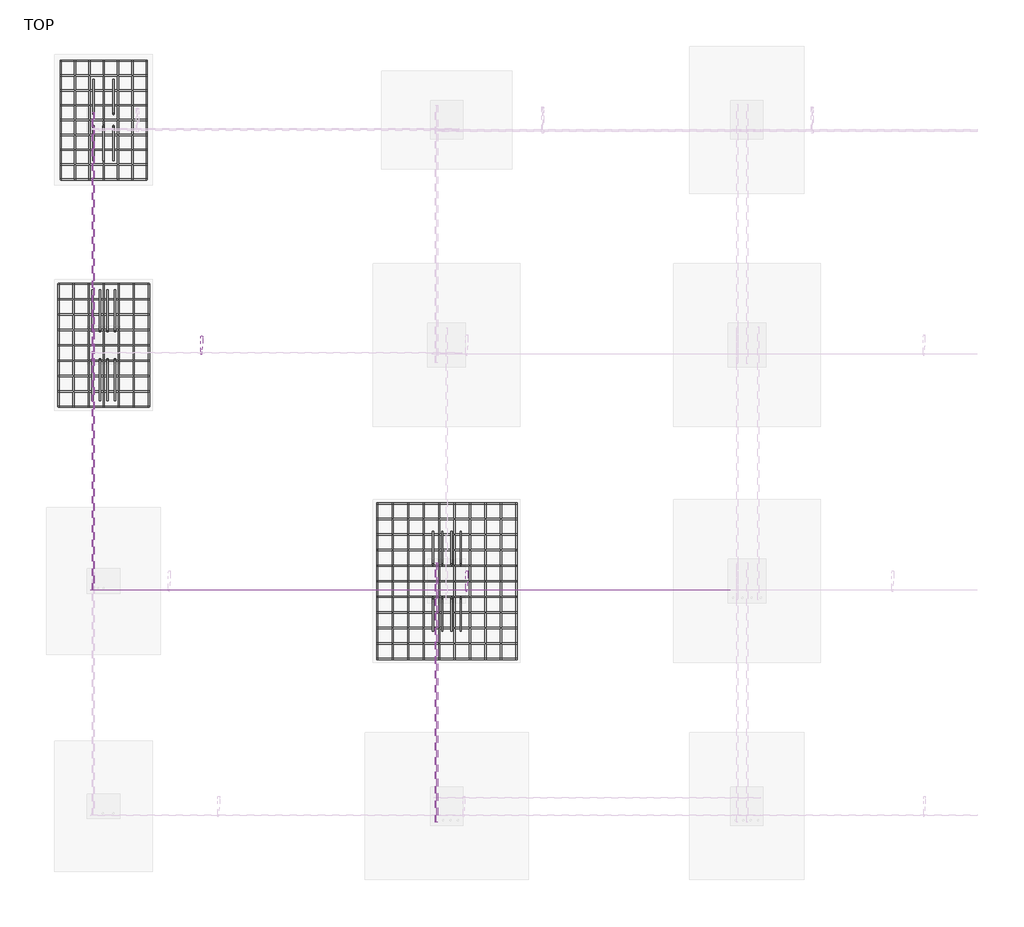
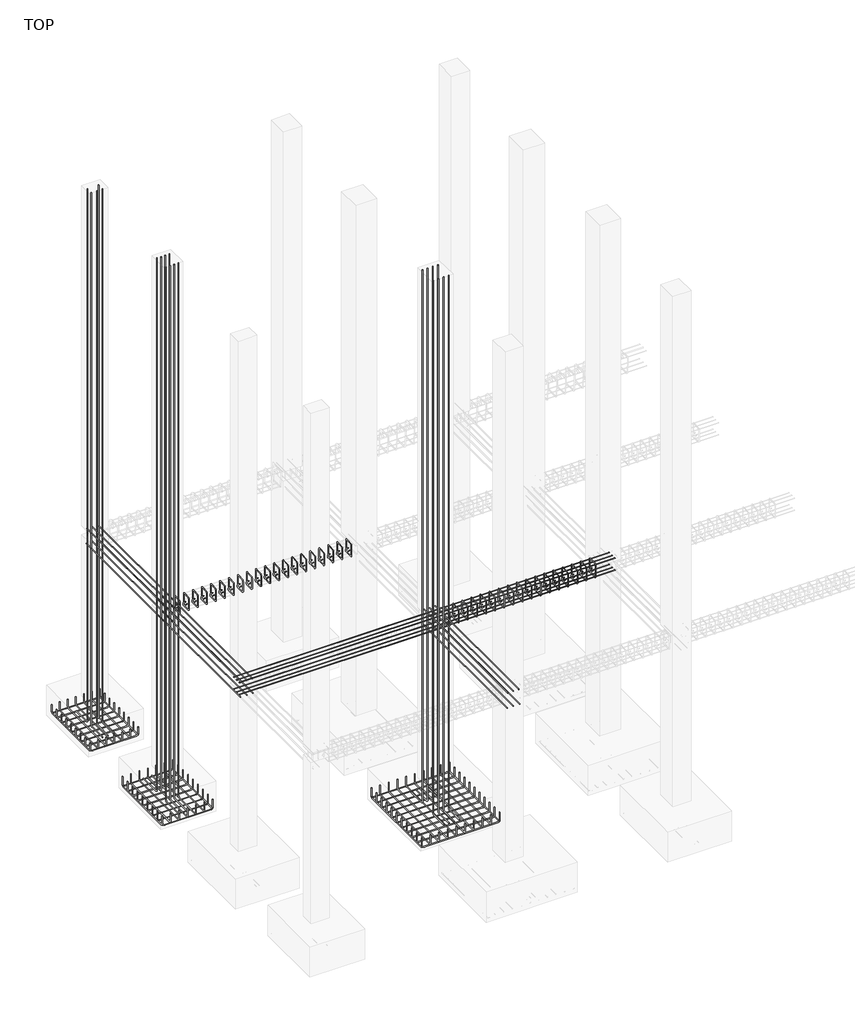
# One storey, part 3 of 8: 24 reinforcing bars.
"""IFC4 building model written with IfcOpenShell, lengths in millimetres."""

from ifc_helpers import new_model, si_unit, point, frame, origin, place, context, project, spatial, polyline, circle_curve, trimmed, segment, composite_curve, source, transform, mapped, element, save
from ifc_brep_helpers import swept_disk

model = new_model("IFC4")

# Units and contexts
model_context = context("Model", 3, world=origin())
ifc_project = project(units=[si_unit("LENGTHUNIT", "METRE", prefix="MILLI")], contexts=[model_context])

# Site, building, storey
site = spatial("IfcSite", under=ifc_project)
building = spatial("IfcBuilding", under=site)
storey = spatial("IfcBuildingStorey", under=building, Name="TOP", Elevation=0.0)

# Reinforcing bars
placement = place(None, origin())
reinforcing_bar_shape = source(origin(), model_context, "Body", "SolidModel", [
    swept_disk(composite_curve([segment(polyline([(-4763.7160601, 8075.5307576, -331.0), (-4763.7160601, 8075.5307576, -447.4)]), True, "CONTINUOUS"), segment(trimmed(circle_curve(frame((-4763.7160601, 8045.5307576, -447.4), z_axis=(-1.0, 0.0, 0.0), x_axis=(0.0, 30.0, 0.0)), 30.0), [point((-4763.7160601, 8075.5307576, -447.4))], [point((-4763.7160601, 8045.5307576, -477.4))], True, "CARTESIAN"), True, "CONTINUOUS"), segment(polyline([(-4763.7160601, 8045.5307576, -477.4), (-4763.7160601, 6998.3307576, -477.4)]), True, "CONTINUOUS"), segment(trimmed(circle_curve(frame((-4763.7160601, 6998.3307576, -447.4), z_axis=(-1.0, 0.0, 0.0), x_axis=(0.0, 0.0, -30.0)), 30.0), [point((-4763.7160601, 6998.3307576, -477.4))], [point((-4763.7160601, 6968.3307576, -447.4))], True, "CARTESIAN"), True, "CONTINUOUS"), segment(polyline([(-4763.7160601, 6968.3307576, -447.4), (-4763.7160601, 6968.3307576, -331.0)]), True, "CONTINUOUS")], self_intersect=False), 6.0),
])
element("IfcReinforcingBar", 1, at=placement, inside=storey, context=model_context, shape_type="MappedRepresentation", body=[
    mapped(reinforcing_bar_shape, transform((0.0, 0.0, 0.0), x_axis=(1.0, 0.0, 0.0), y_axis=(0.0, 1.0, 0.0), z_axis=(0.0, 0.0, 1.0))),
    mapped(reinforcing_bar_shape, transform((-133.7333333, 0.0, 0.0), x_axis=(1.0, 0.0, 0.0), y_axis=(0.0, 1.0, 0.0), z_axis=(0.0, 0.0, 1.0))),
    mapped(reinforcing_bar_shape, transform((-267.4666667, 0.0, 0.0), x_axis=(1.0, 0.0, 0.0), y_axis=(0.0, 1.0, 0.0), z_axis=(0.0, 0.0, 1.0))),
    mapped(reinforcing_bar_shape, transform((-401.2, 0.0, 0.0), x_axis=(1.0, 0.0, 0.0), y_axis=(0.0, 1.0, 0.0), z_axis=(0.0, 0.0, 1.0))),
    mapped(reinforcing_bar_shape, transform((-534.9333333, 0.0, 0.0), x_axis=(1.0, 0.0, 0.0), y_axis=(0.0, 1.0, 0.0), z_axis=(0.0, 0.0, 1.0))),
    mapped(reinforcing_bar_shape, transform((-668.6666667, 0.0, 0.0), x_axis=(1.0, 0.0, 0.0), y_axis=(0.0, 1.0, 0.0), z_axis=(0.0, 0.0, 1.0))),
    mapped(reinforcing_bar_shape, transform((-802.4, 0.0, 0.0), x_axis=(1.0, 0.0, 0.0), y_axis=(0.0, 1.0, 0.0), z_axis=(0.0, 0.0, 1.0))),
])
reinforcing_bar_2_shape = source(origin(), model_context, "Body", "SolidModel", [
    swept_disk(composite_curve([segment(polyline([(-5566.1160601, 8075.5307576, -331.0), (-5566.1160601, 8075.5307576, -447.4)]), True, "CONTINUOUS"), segment(trimmed(circle_curve(frame((-5536.1160601, 8075.5307576, -447.4), z_axis=(0.0, -1.0, 0.0), x_axis=(-30.0, 0.0, 0.0)), 30.0), [point((-5566.1160601, 8075.5307576, -447.4))], [point((-5536.1160601, 8075.5307576, -477.4))], True, "CARTESIAN"), True, "CONTINUOUS"), segment(polyline([(-5536.1160601, 8075.5307576, -477.4), (-4793.7160601, 8075.5307576, -477.4)]), True, "CONTINUOUS"), segment(trimmed(circle_curve(frame((-4793.7160601, 8075.5307576, -447.4), z_axis=(0.0, -1.0, 0.0), x_axis=(0.0, 0.0, -30.0)), 30.0), [point((-4793.7160601, 8075.5307576, -477.4))], [point((-4763.7160601, 8075.5307576, -447.4))], True, "CARTESIAN"), True, "CONTINUOUS"), segment(polyline([(-4763.7160601, 8075.5307576, -447.4), (-4763.7160601, 8075.5307576, -331.0)]), True, "CONTINUOUS")], self_intersect=False), 6.0),
])
element("IfcReinforcingBar", 2, at=placement, inside=storey, context=model_context, shape_type="MappedRepresentation", body=[
    mapped(reinforcing_bar_2_shape, transform((0.0, 0.0, 0.0), x_axis=(1.0, 0.0, 0.0), y_axis=(0.0, 1.0, 0.0), z_axis=(0.0, 0.0, 1.0))),
    mapped(reinforcing_bar_2_shape, transform((0.0, -138.4, 0.0), x_axis=(1.0, 0.0, 0.0), y_axis=(0.0, 1.0, 0.0), z_axis=(0.0, 0.0, 1.0))),
    mapped(reinforcing_bar_2_shape, transform((0.0, -276.8, 0.0), x_axis=(1.0, 0.0, 0.0), y_axis=(0.0, 1.0, 0.0), z_axis=(0.0, 0.0, 1.0))),
    mapped(reinforcing_bar_2_shape, transform((0.0, -415.2, 0.0), x_axis=(1.0, 0.0, 0.0), y_axis=(0.0, 1.0, 0.0), z_axis=(0.0, 0.0, 1.0))),
    mapped(reinforcing_bar_2_shape, transform((0.0, -553.6, 0.0), x_axis=(1.0, 0.0, 0.0), y_axis=(0.0, 1.0, 0.0), z_axis=(0.0, 0.0, 1.0))),
    mapped(reinforcing_bar_2_shape, transform((0.0, -692.0, 0.0), x_axis=(1.0, 0.0, 0.0), y_axis=(0.0, 1.0, 0.0), z_axis=(0.0, 0.0, 1.0))),
    mapped(reinforcing_bar_2_shape, transform((0.0, -830.4, 0.0), x_axis=(1.0, 0.0, 0.0), y_axis=(0.0, 1.0, 0.0), z_axis=(0.0, 0.0, 1.0))),
    mapped(reinforcing_bar_2_shape, transform((0.0, -968.8, 0.0), x_axis=(1.0, 0.0, 0.0), y_axis=(0.0, 1.0, 0.0), z_axis=(0.0, 0.0, 1.0))),
    mapped(reinforcing_bar_2_shape, transform((0.0, -1107.2, 0.0), x_axis=(1.0, 0.0, 0.0), y_axis=(0.0, 1.0, 0.0), z_axis=(0.0, 0.0, 1.0))),
])
reinforcing_bar_3_shape = source(origin(), model_context, "Body", "SolidModel", [
    swept_disk(composite_curve([segment(polyline([(-5259.3160601, 7577.9568407, 8958.464), (-5259.3160601, 7577.9568407, -415.886)]), True, "CONTINUOUS"), segment(trimmed(circle_curve(frame((-5259.3160601, 7607.9568407, -415.886), z_axis=(1.0, 0.0, 0.0), x_axis=(0.0, -30.0, 0.0)), 30.0), [point((-5259.3160601, 7577.9568407, -415.886))], [point((-5259.3160601, 7607.9568407, -445.886))], True, "CARTESIAN"), True, "CONTINUOUS"), segment(polyline([(-5259.3160601, 7607.9568407, -445.886), (-5259.3160601, 7901.0307576, -445.886)]), True, "CONTINUOUS")], self_intersect=False), 6.0),
])
element("IfcReinforcingBar", 3, at=placement, inside=storey, context=model_context, shape_type="MappedRepresentation", body=[
    mapped(reinforcing_bar_3_shape, transform((0.0, 0.0, 0.0), x_axis=(1.0, 0.0, 0.0), y_axis=(0.0, 1.0, 0.0), z_axis=(0.0, 0.0, 1.0))),
    mapped(reinforcing_bar_3_shape, transform((185.9681172, 0.0, 0.0), x_axis=(1.0, 0.0, 0.0), y_axis=(0.0, 1.0, 0.0), z_axis=(0.0, 0.0, 1.0))),
])
reinforcing_bar_4_shape = source(origin(), model_context, "Body", "SolidModel", [
    swept_disk(composite_curve([segment(polyline([(-5073.3479429, 7465.6307576, 8958.464), (-5073.3479429, 7465.6307576, -415.886)]), True, "CONTINUOUS"), segment(trimmed(circle_curve(frame((-5073.3479429, 7435.6307576, -415.886), z_axis=(-1.0, 0.0, 0.0), x_axis=(0.0, 30.0, 0.0)), 30.0), [point((-5073.3479429, 7465.6307576, -415.886))], [point((-5073.3479429, 7435.6307576, -445.886))], True, "CARTESIAN"), True, "CONTINUOUS"), segment(polyline([(-5073.3479429, 7435.6307576, -445.886), (-5073.3479429, 7142.8307576, -445.886)]), True, "CONTINUOUS")], self_intersect=False), 6.0),
])
element("IfcReinforcingBar", 4, at=placement, inside=storey, context=model_context, shape_type="MappedRepresentation", body=[
    mapped(reinforcing_bar_4_shape, transform((0.0, 0.0, 0.0), x_axis=(1.0, 0.0, 0.0), y_axis=(0.0, 1.0, 0.0), z_axis=(0.0, 0.0, 1.0))),
    mapped(reinforcing_bar_4_shape, transform((-92.9840586, 0.0, 0.0), x_axis=(1.0, 0.0, 0.0), y_axis=(0.0, 1.0, 0.0), z_axis=(0.0, 0.0, 1.0))),
    mapped(reinforcing_bar_4_shape, transform((-185.9681172, 0.0, 0.0), x_axis=(1.0, 0.0, 0.0), y_axis=(0.0, 1.0, 0.0), z_axis=(0.0, 0.0, 1.0))),
])
reinforcing_bar_5_shape = source(origin(), model_context, "Body", "SolidModel", [
    swept_disk(composite_curve([segment(polyline([(-4743.7160601, 5995.5307576, -331.0), (-4743.7160601, 5995.5307576, -467.4)]), True, "CONTINUOUS"), segment(trimmed(circle_curve(frame((-4743.7160601, 5965.5307576, -467.4), z_axis=(-1.0, 0.0, 0.0), x_axis=(0.0, 30.0, 0.0)), 30.0), [point((-4743.7160601, 5995.5307576, -467.4))], [point((-4743.7160601, 5965.5307576, -497.4))], True, "CARTESIAN"), True, "CONTINUOUS"), segment(polyline([(-4743.7160601, 5965.5307576, -497.4), (-4743.7160601, 4878.3307576, -497.4)]), True, "CONTINUOUS"), segment(trimmed(circle_curve(frame((-4743.7160601, 4878.3307576, -467.4), z_axis=(-1.0, 0.0, 0.0), x_axis=(0.0, 0.0, -30.0)), 30.0), [point((-4743.7160601, 4878.3307576, -497.4))], [point((-4743.7160601, 4848.3307576, -467.4))], True, "CARTESIAN"), True, "CONTINUOUS"), segment(polyline([(-4743.7160601, 4848.3307576, -467.4), (-4743.7160601, 4848.3307576, -331.0)]), True, "CONTINUOUS")], self_intersect=False), 6.0),
])
element("IfcReinforcingBar", 5, at=placement, inside=storey, context=model_context, shape_type="MappedRepresentation", body=[
    mapped(reinforcing_bar_5_shape, transform((0.0, 0.0, 0.0), x_axis=(1.0, 0.0, 0.0), y_axis=(0.0, 1.0, 0.0), z_axis=(0.0, 0.0, 1.0))),
    mapped(reinforcing_bar_5_shape, transform((-140.4, 0.0, 0.0), x_axis=(1.0, 0.0, 0.0), y_axis=(0.0, 1.0, 0.0), z_axis=(0.0, 0.0, 1.0))),
    mapped(reinforcing_bar_5_shape, transform((-280.8, 0.0, 0.0), x_axis=(1.0, 0.0, 0.0), y_axis=(0.0, 1.0, 0.0), z_axis=(0.0, 0.0, 1.0))),
    mapped(reinforcing_bar_5_shape, transform((-421.2, 0.0, 0.0), x_axis=(1.0, 0.0, 0.0), y_axis=(0.0, 1.0, 0.0), z_axis=(0.0, 0.0, 1.0))),
    mapped(reinforcing_bar_5_shape, transform((-561.6, 0.0, 0.0), x_axis=(1.0, 0.0, 0.0), y_axis=(0.0, 1.0, 0.0), z_axis=(0.0, 0.0, 1.0))),
    mapped(reinforcing_bar_5_shape, transform((-702.0, 0.0, 0.0), x_axis=(1.0, 0.0, 0.0), y_axis=(0.0, 1.0, 0.0), z_axis=(0.0, 0.0, 1.0))),
    mapped(reinforcing_bar_5_shape, transform((-842.4, 0.0, 0.0), x_axis=(1.0, 0.0, 0.0), y_axis=(0.0, 1.0, 0.0), z_axis=(0.0, 0.0, 1.0))),
])
reinforcing_bar_6_shape = source(origin(), model_context, "Body", "SolidModel", [
    swept_disk(composite_curve([segment(polyline([(-5586.1160601, 5995.5307576, -331.0), (-5586.1160601, 5995.5307576, -467.4)]), True, "CONTINUOUS"), segment(trimmed(circle_curve(frame((-5556.1160601, 5995.5307576, -467.4), z_axis=(0.0, -1.0, 0.0), x_axis=(-30.0, 0.0, 0.0)), 30.0), [point((-5586.1160601, 5995.5307576, -467.4))], [point((-5556.1160601, 5995.5307576, -497.4))], True, "CARTESIAN"), True, "CONTINUOUS"), segment(polyline([(-5556.1160601, 5995.5307576, -497.4), (-4773.7160601, 5995.5307576, -497.4)]), True, "CONTINUOUS"), segment(trimmed(circle_curve(frame((-4773.7160601, 5995.5307576, -467.4), z_axis=(0.0, -1.0, 0.0), x_axis=(0.0, 0.0, -30.0)), 30.0), [point((-4773.7160601, 5995.5307576, -497.4))], [point((-4743.7160601, 5995.5307576, -467.4))], True, "CARTESIAN"), True, "CONTINUOUS"), segment(polyline([(-4743.7160601, 5995.5307576, -467.4), (-4743.7160601, 5995.5307576, -331.0)]), True, "CONTINUOUS")], self_intersect=False), 6.0),
])
element("IfcReinforcingBar", 6, at=placement, inside=storey, context=model_context, shape_type="MappedRepresentation", body=[
    mapped(reinforcing_bar_6_shape, transform((0.0, 0.0, 0.0), x_axis=(1.0, 0.0, 0.0), y_axis=(0.0, 1.0, 0.0), z_axis=(0.0, 0.0, 1.0))),
    mapped(reinforcing_bar_6_shape, transform((0.0, -143.4, 0.0), x_axis=(1.0, 0.0, 0.0), y_axis=(0.0, 1.0, 0.0), z_axis=(0.0, 0.0, 1.0))),
    mapped(reinforcing_bar_6_shape, transform((0.0, -286.8, 0.0), x_axis=(1.0, 0.0, 0.0), y_axis=(0.0, 1.0, 0.0), z_axis=(0.0, 0.0, 1.0))),
    mapped(reinforcing_bar_6_shape, transform((0.0, -430.2, 0.0), x_axis=(1.0, 0.0, 0.0), y_axis=(0.0, 1.0, 0.0), z_axis=(0.0, 0.0, 1.0))),
    mapped(reinforcing_bar_6_shape, transform((0.0, -573.6, 0.0), x_axis=(1.0, 0.0, 0.0), y_axis=(0.0, 1.0, 0.0), z_axis=(0.0, 0.0, 1.0))),
    mapped(reinforcing_bar_6_shape, transform((0.0, -717.0, 0.0), x_axis=(1.0, 0.0, 0.0), y_axis=(0.0, 1.0, 0.0), z_axis=(0.0, 0.0, 1.0))),
    mapped(reinforcing_bar_6_shape, transform((0.0, -860.4, 0.0), x_axis=(1.0, 0.0, 0.0), y_axis=(0.0, 1.0, 0.0), z_axis=(0.0, 0.0, 1.0))),
    mapped(reinforcing_bar_6_shape, transform((0.0, -1003.8, 0.0), x_axis=(1.0, 0.0, 0.0), y_axis=(0.0, 1.0, 0.0), z_axis=(0.0, 0.0, 1.0))),
    mapped(reinforcing_bar_6_shape, transform((0.0, -1147.2, 0.0), x_axis=(1.0, 0.0, 0.0), y_axis=(0.0, 1.0, 0.0), z_axis=(0.0, 0.0, 1.0))),
])
reinforcing_bar_7_shape = source(origin(), model_context, "Body", "SolidModel", [
    swept_disk(composite_curve([segment(polyline([(-5269.3160601, 5551.7815576, 8968.464), (-5269.3160601, 5551.7815576, -409.536)]), True, "CONTINUOUS"), segment(trimmed(circle_curve(frame((-5269.3160601, 5581.7815576, -409.536), z_axis=(1.0, 0.0, 0.0), x_axis=(0.0, -30.0, 0.0)), 30.0), [point((-5269.3160601, 5551.7815576, -409.536))], [point((-5269.3160601, 5581.7815576, -439.536))], True, "CARTESIAN"), True, "CONTINUOUS"), segment(polyline([(-5269.3160601, 5581.7815576, -439.536), (-5269.3160601, 5940.7815576, -439.536)]), True, "CONTINUOUS")], self_intersect=False), 6.0),
])
element("IfcReinforcingBar", 7, at=placement, inside=storey, context=model_context, shape_type="MappedRepresentation", body=[
    mapped(reinforcing_bar_7_shape, transform((0.0, 0.0, 0.0), x_axis=(1.0, 0.0, 0.0), y_axis=(0.0, 1.0, 0.0), z_axis=(0.0, 0.0, 1.0))),
    mapped(reinforcing_bar_7_shape, transform((69.6, 0.0, 0.0), x_axis=(1.0, 0.0, 0.0), y_axis=(0.0, 1.0, 0.0), z_axis=(0.0, 0.0, 1.0))),
    mapped(reinforcing_bar_7_shape, transform((139.2, 0.0, 0.0), x_axis=(1.0, 0.0, 0.0), y_axis=(0.0, 1.0, 0.0), z_axis=(0.0, 0.0, 1.0))),
    mapped(reinforcing_bar_7_shape, transform((208.8, 0.0, 0.0), x_axis=(1.0, 0.0, 0.0), y_axis=(0.0, 1.0, 0.0), z_axis=(0.0, 0.0, 1.0))),
])
reinforcing_bar_8_shape = source(origin(), model_context, "Body", "SolidModel", [
    swept_disk(composite_curve([segment(polyline([(-5060.5160601, 5292.0799576, 8968.464), (-5060.5160601, 5292.0799576, -415.886)]), True, "CONTINUOUS"), segment(trimmed(circle_curve(frame((-5060.5160601, 5262.0799576, -415.886), z_axis=(-1.0, 0.0, 0.0), x_axis=(0.0, 30.0, 0.0)), 30.0), [point((-5060.5160601, 5292.0799576, -415.886))], [point((-5060.5160601, 5262.0799576, -445.886))], True, "CARTESIAN"), True, "CONTINUOUS"), segment(polyline([(-5060.5160601, 5262.0799576, -445.886), (-5060.5160601, 4903.0799576, -445.886)]), True, "CONTINUOUS")], self_intersect=False), 6.0),
])
element("IfcReinforcingBar", 8, at=placement, inside=storey, context=model_context, shape_type="MappedRepresentation", body=[
    mapped(reinforcing_bar_8_shape, transform((0.0, 0.0, 0.0), x_axis=(1.0, 0.0, 0.0), y_axis=(0.0, 1.0, 0.0), z_axis=(0.0, 0.0, 1.0))),
    mapped(reinforcing_bar_8_shape, transform((-69.6, 0.0, 0.0), x_axis=(1.0, 0.0, 0.0), y_axis=(0.0, 1.0, 0.0), z_axis=(0.0, 0.0, 1.0))),
    mapped(reinforcing_bar_8_shape, transform((-139.2, 0.0, 0.0), x_axis=(1.0, 0.0, 0.0), y_axis=(0.0, 1.0, 0.0), z_axis=(0.0, 0.0, 1.0))),
    mapped(reinforcing_bar_8_shape, transform((-208.8, 0.0, 0.0), x_axis=(1.0, 0.0, 0.0), y_axis=(0.0, 1.0, 0.0), z_axis=(0.0, 0.0, 1.0))),
])
reinforcing_bar_9_shape = source(origin(), model_context, "Body", "SolidModel", [
    swept_disk(composite_curve([segment(polyline([(-2094.7668601, 3376.2799576, 8968.464), (-2094.7668601, 3376.2799576, -403.186)]), True, "CONTINUOUS"), segment(trimmed(circle_curve(frame((-2094.7668601, 3406.2799576, -403.186), z_axis=(1.0, 0.0, 0.0), x_axis=(0.0, -30.0, 0.0)), 30.0), [point((-2094.7668601, 3376.2799576, -403.186))], [point((-2094.7668601, 3406.2799576, -433.186))], True, "CARTESIAN"), True, "CONTINUOUS"), segment(polyline([(-2094.7668601, 3406.2799576, -433.186), (-2094.7668601, 3689.0799576, -433.186)]), True, "CONTINUOUS")], self_intersect=False), 6.0),
])
element("IfcReinforcingBar", 9, at=placement, inside=storey, context=model_context, shape_type="MappedRepresentation", body=[
    mapped(reinforcing_bar_9_shape, transform((0.0, 0.0, 0.0), x_axis=(1.0, 0.0, 0.0), y_axis=(0.0, 1.0, 0.0), z_axis=(0.0, 0.0, 1.0))),
    mapped(reinforcing_bar_9_shape, transform((86.5672, 0.0, 0.0), x_axis=(1.0, 0.0, 0.0), y_axis=(0.0, 1.0, 0.0), z_axis=(0.0, 0.0, 1.0))),
    mapped(reinforcing_bar_9_shape, transform((173.1344, 0.0, 0.0), x_axis=(1.0, 0.0, 0.0), y_axis=(0.0, 1.0, 0.0), z_axis=(0.0, 0.0, 1.0))),
    mapped(reinforcing_bar_9_shape, transform((259.7016, 0.0, 0.0), x_axis=(1.0, 0.0, 0.0), y_axis=(0.0, 1.0, 0.0), z_axis=(0.0, 0.0, 1.0))),
])
reinforcing_bar_10_shape = source(origin(), model_context, "Body", "SolidModel", [
    swept_disk(composite_curve([segment(polyline([(-1835.0652601, 3065.9815576, 8968.464), (-1835.0652601, 3065.9815576, -409.536)]), True, "CONTINUOUS"), segment(trimmed(circle_curve(frame((-1835.0652601, 3035.9815576, -409.536), z_axis=(-1.0, 0.0, 0.0), x_axis=(0.0, 30.0, 0.0)), 30.0), [point((-1835.0652601, 3065.9815576, -409.536))], [point((-1835.0652601, 3035.9815576, -439.536))], True, "CARTESIAN"), True, "CONTINUOUS"), segment(polyline([(-1835.0652601, 3035.9815576, -439.536), (-1835.0652601, 2753.1815576, -439.536)]), True, "CONTINUOUS")], self_intersect=False), 6.0),
])
element("IfcReinforcingBar", 10, at=placement, inside=storey, context=model_context, shape_type="MappedRepresentation", body=[
    mapped(reinforcing_bar_10_shape, transform((0.0, 0.0, 0.0), x_axis=(1.0, 0.0, 0.0), y_axis=(0.0, 1.0, 0.0), z_axis=(0.0, 0.0, 1.0))),
    mapped(reinforcing_bar_10_shape, transform((-86.5672, 0.0, 0.0), x_axis=(1.0, 0.0, 0.0), y_axis=(0.0, 1.0, 0.0), z_axis=(0.0, 0.0, 1.0))),
    mapped(reinforcing_bar_10_shape, transform((-173.1344, 0.0, 0.0), x_axis=(1.0, 0.0, 0.0), y_axis=(0.0, 1.0, 0.0), z_axis=(0.0, 0.0, 1.0))),
    mapped(reinforcing_bar_10_shape, transform((-259.7016, 0.0, 0.0), x_axis=(1.0, 0.0, 0.0), y_axis=(0.0, 1.0, 0.0), z_axis=(0.0, 0.0, 1.0))),
])
reinforcing_bar_11_shape = source(origin(), model_context, "Body", "SolidModel", [
    swept_disk(composite_curve([segment(polyline([(-2614.7160601, 3947.1307576, -331.0), (-2614.7160601, 3947.1307576, -467.4)]), True, "CONTINUOUS"), segment(trimmed(circle_curve(frame((-2584.7160601, 3947.1307576, -467.4), z_axis=(0.0, -1.0, 0.0), x_axis=(-30.0, 0.0, 0.0)), 30.0), [point((-2614.7160601, 3947.1307576, -467.4))], [point((-2584.7160601, 3947.1307576, -497.4))], True, "CARTESIAN"), True, "CONTINUOUS"), segment(polyline([(-2584.7160601, 3947.1307576, -497.4), (-1345.1160601, 3947.1307576, -497.4)]), True, "CONTINUOUS"), segment(trimmed(circle_curve(frame((-1345.1160601, 3947.1307576, -467.4), z_axis=(0.0, -1.0, 0.0), x_axis=(0.0, 0.0, -30.0)), 30.0), [point((-1345.1160601, 3947.1307576, -497.4))], [point((-1315.1160601, 3947.1307576, -467.4))], True, "CARTESIAN"), True, "CONTINUOUS"), segment(polyline([(-1315.1160601, 3947.1307576, -467.4), (-1315.1160601, 3947.1307576, -331.0)]), True, "CONTINUOUS")], self_intersect=False), 6.0),
])
element("IfcReinforcingBar", 11, at=placement, inside=storey, context=model_context, shape_type="MappedRepresentation", body=[
    mapped(reinforcing_bar_11_shape, transform((0.0, 0.0, 0.0), x_axis=(1.0, 0.0, 0.0), y_axis=(0.0, 1.0, 0.0), z_axis=(0.0, 0.0, 1.0))),
    mapped(reinforcing_bar_11_shape, transform((0.0, -145.2, 0.0), x_axis=(1.0, 0.0, 0.0), y_axis=(0.0, 1.0, 0.0), z_axis=(0.0, 0.0, 1.0))),
    mapped(reinforcing_bar_11_shape, transform((0.0, -290.4, 0.0), x_axis=(1.0, 0.0, 0.0), y_axis=(0.0, 1.0, 0.0), z_axis=(0.0, 0.0, 1.0))),
    mapped(reinforcing_bar_11_shape, transform((0.0, -435.6, 0.0), x_axis=(1.0, 0.0, 0.0), y_axis=(0.0, 1.0, 0.0), z_axis=(0.0, 0.0, 1.0))),
    mapped(reinforcing_bar_11_shape, transform((0.0, -580.8, 0.0), x_axis=(1.0, 0.0, 0.0), y_axis=(0.0, 1.0, 0.0), z_axis=(0.0, 0.0, 1.0))),
    mapped(reinforcing_bar_11_shape, transform((0.0, -726.0, 0.0), x_axis=(1.0, 0.0, 0.0), y_axis=(0.0, 1.0, 0.0), z_axis=(0.0, 0.0, 1.0))),
    mapped(reinforcing_bar_11_shape, transform((0.0, -871.2, 0.0), x_axis=(1.0, 0.0, 0.0), y_axis=(0.0, 1.0, 0.0), z_axis=(0.0, 0.0, 1.0))),
    mapped(reinforcing_bar_11_shape, transform((0.0, -1016.4, 0.0), x_axis=(1.0, 0.0, 0.0), y_axis=(0.0, 1.0, 0.0), z_axis=(0.0, 0.0, 1.0))),
    mapped(reinforcing_bar_11_shape, transform((0.0, -1161.6, 0.0), x_axis=(1.0, 0.0, 0.0), y_axis=(0.0, 1.0, 0.0), z_axis=(0.0, 0.0, 1.0))),
    mapped(reinforcing_bar_11_shape, transform((0.0, -1306.8, 0.0), x_axis=(1.0, 0.0, 0.0), y_axis=(0.0, 1.0, 0.0), z_axis=(0.0, 0.0, 1.0))),
    mapped(reinforcing_bar_11_shape, transform((0.0, -1452.0, 0.0), x_axis=(1.0, 0.0, 0.0), y_axis=(0.0, 1.0, 0.0), z_axis=(0.0, 0.0, 1.0))),
])
reinforcing_bar_12_shape = source(origin(), model_context, "Body", "SolidModel", [
    swept_disk(composite_curve([segment(polyline([(-2614.7160601, 2495.1307576, -331.0), (-2614.7160601, 2495.1307576, -467.4)]), True, "CONTINUOUS"), segment(trimmed(circle_curve(frame((-2614.7160601, 2525.1307576, -467.4), z_axis=(1.0, 0.0, 0.0), x_axis=(0.0, -30.0, 0.0)), 30.0), [point((-2614.7160601, 2495.1307576, -467.4))], [point((-2614.7160601, 2525.1307576, -497.4))], True, "CARTESIAN"), True, "CONTINUOUS"), segment(polyline([(-2614.7160601, 2525.1307576, -497.4), (-2614.7160601, 3917.1307576, -497.4)]), True, "CONTINUOUS"), segment(trimmed(circle_curve(frame((-2614.7160601, 3917.1307576, -467.4), z_axis=(1.0, 0.0, 0.0), x_axis=(0.0, 0.0, -30.0)), 30.0), [point((-2614.7160601, 3917.1307576, -497.4))], [point((-2614.7160601, 3947.1307576, -467.4))], True, "CARTESIAN"), True, "CONTINUOUS"), segment(polyline([(-2614.7160601, 3947.1307576, -467.4), (-2614.7160601, 3947.1307576, -331.0)]), True, "CONTINUOUS")], self_intersect=False), 6.0),
])
element("IfcReinforcingBar", 12, at=placement, inside=storey, context=model_context, shape_type="MappedRepresentation", body=[
    mapped(reinforcing_bar_12_shape, transform((0.0, 0.0, 0.0), x_axis=(1.0, 0.0, 0.0), y_axis=(0.0, 1.0, 0.0), z_axis=(0.0, 0.0, 1.0))),
    mapped(reinforcing_bar_12_shape, transform((144.4, 0.0, 0.0), x_axis=(1.0, 0.0, 0.0), y_axis=(0.0, 1.0, 0.0), z_axis=(0.0, 0.0, 1.0))),
    mapped(reinforcing_bar_12_shape, transform((288.8, 0.0, 0.0), x_axis=(1.0, 0.0, 0.0), y_axis=(0.0, 1.0, 0.0), z_axis=(0.0, 0.0, 1.0))),
    mapped(reinforcing_bar_12_shape, transform((433.2, 0.0, 0.0), x_axis=(1.0, 0.0, 0.0), y_axis=(0.0, 1.0, 0.0), z_axis=(0.0, 0.0, 1.0))),
    mapped(reinforcing_bar_12_shape, transform((577.6, 0.0, 0.0), x_axis=(1.0, 0.0, 0.0), y_axis=(0.0, 1.0, 0.0), z_axis=(0.0, 0.0, 1.0))),
    mapped(reinforcing_bar_12_shape, transform((722.0, 0.0, 0.0), x_axis=(1.0, 0.0, 0.0), y_axis=(0.0, 1.0, 0.0), z_axis=(0.0, 0.0, 1.0))),
    mapped(reinforcing_bar_12_shape, transform((866.4, 0.0, 0.0), x_axis=(1.0, 0.0, 0.0), y_axis=(0.0, 1.0, 0.0), z_axis=(0.0, 0.0, 1.0))),
    mapped(reinforcing_bar_12_shape, transform((1010.8, 0.0, 0.0), x_axis=(1.0, 0.0, 0.0), y_axis=(0.0, 1.0, 0.0), z_axis=(0.0, 0.0, 1.0))),
    mapped(reinforcing_bar_12_shape, transform((1155.2, 0.0, 0.0), x_axis=(1.0, 0.0, 0.0), y_axis=(0.0, 1.0, 0.0), z_axis=(0.0, 0.0, 1.0))),
    mapped(reinforcing_bar_12_shape, transform((1299.6, 0.0, 0.0), x_axis=(1.0, 0.0, 0.0), y_axis=(0.0, 1.0, 0.0), z_axis=(0.0, 0.0, 1.0))),
])
reinforcing_bar_13_shape = source(origin(), model_context, "Body", "SolidModel", [
    swept_disk(composite_curve([segment(polyline([(-5267.9226618, 7596.2307576, 2693.6917983), (-5267.9226618, 5274.0799576, 2693.6917983)]), True, "CONTINUOUS")], self_intersect=False), 5.0),
])
element("IfcReinforcingBar", 13, at=placement, inside=storey, context=model_context, shape_type="MappedRepresentation", body=[
    mapped(reinforcing_bar_13_shape, transform((0.0, 0.0, 0.0), x_axis=(1.0, 0.0, 0.0), y_axis=(0.0, 1.0, 0.0), z_axis=(0.0, 0.0, 1.0))),
    mapped(reinforcing_bar_13_shape, transform((103.0066017, 0.0, 0.0), x_axis=(1.0, 0.0, 0.0), y_axis=(0.0, 1.0, 0.0), z_axis=(0.0, 0.0, 1.0))),
    mapped(reinforcing_bar_13_shape, transform((206.0132034, 0.0, 0.0), x_axis=(1.0, 0.0, 0.0), y_axis=(0.0, 1.0, 0.0), z_axis=(0.0, 0.0, 1.0))),
])
reinforcing_bar_14_shape = source(origin(), model_context, "Body", "SolidModel", [
    swept_disk(composite_curve([segment(polyline([(-5257.3160601, 5274.0799576, 2955.0), (-5257.3160601, 7596.2307576, 2955.0)]), True, "CONTINUOUS")], self_intersect=False), 5.0),
])
element("IfcReinforcingBar", 14, at=placement, inside=storey, context=model_context, shape_type="MappedRepresentation", body=[
    mapped(reinforcing_bar_14_shape, transform((0.0, 0.0, 0.0), x_axis=(1.0, 0.0, 0.0), y_axis=(0.0, 1.0, 0.0), z_axis=(0.0, 0.0, 1.0))),
    mapped(reinforcing_bar_14_shape, transform((92.4, 0.0, 0.0), x_axis=(1.0, 0.0, 0.0), y_axis=(0.0, 1.0, 0.0), z_axis=(0.0, 0.0, 1.0))),
    mapped(reinforcing_bar_14_shape, transform((184.8, 0.0, 0.0), x_axis=(1.0, 0.0, 0.0), y_axis=(0.0, 1.0, 0.0), z_axis=(0.0, 0.0, 1.0))),
])
reinforcing_bar_15_shape = source(origin(), model_context, "Body", "SolidModel", [
    swept_disk(composite_curve([segment(polyline([(-5267.9226618, 5569.7815576, 2693.6917983), (-5267.9226618, 3136.8307576, 2693.6917983)]), True, "CONTINUOUS")], self_intersect=False), 5.0),
])
element("IfcReinforcingBar", 15, at=placement, inside=storey, context=model_context, shape_type="MappedRepresentation", body=[
    mapped(reinforcing_bar_15_shape, transform((0.0, 0.0, 0.0), x_axis=(1.0, 0.0, 0.0), y_axis=(0.0, 1.0, 0.0), z_axis=(0.0, 0.0, 1.0))),
    mapped(reinforcing_bar_15_shape, transform((103.0066017, 0.0, 0.0), x_axis=(1.0, 0.0, 0.0), y_axis=(0.0, 1.0, 0.0), z_axis=(0.0, 0.0, 1.0))),
    mapped(reinforcing_bar_15_shape, transform((206.0132034, 0.0, 0.0), x_axis=(1.0, 0.0, 0.0), y_axis=(0.0, 1.0, 0.0), z_axis=(0.0, 0.0, 1.0))),
])
reinforcing_bar_16_shape = source(origin(), model_context, "Body", "SolidModel", [
    swept_disk(composite_curve([segment(polyline([(-5257.3160601, 3136.8307576, 2955.0), (-5257.3160601, 5569.7815576, 2955.0)]), True, "CONTINUOUS")], self_intersect=False), 5.0),
])
element("IfcReinforcingBar", 16, at=placement, inside=storey, context=model_context, shape_type="MappedRepresentation", body=[
    mapped(reinforcing_bar_16_shape, transform((0.0, 0.0, 0.0), x_axis=(1.0, 0.0, 0.0), y_axis=(0.0, 1.0, 0.0), z_axis=(0.0, 0.0, 1.0))),
    mapped(reinforcing_bar_16_shape, transform((92.4, 0.0, 0.0), x_axis=(1.0, 0.0, 0.0), y_axis=(0.0, 1.0, 0.0), z_axis=(0.0, 0.0, 1.0))),
    mapped(reinforcing_bar_16_shape, transform((184.8, 0.0, 0.0), x_axis=(1.0, 0.0, 0.0), y_axis=(0.0, 1.0, 0.0), z_axis=(0.0, 0.0, 1.0))),
])
reinforcing_bar_17_shape = source(origin(), model_context, "Body", "SolidModel", [
    swept_disk(composite_curve([segment(polyline([(-2067.9226618, 3394.2799576, 2693.6917983), (-2067.9226618, 973.2799576, 2693.6917983)]), True, "CONTINUOUS")], self_intersect=False), 5.0),
])
element("IfcReinforcingBar", 17, at=placement, inside=storey, context=model_context, shape_type="MappedRepresentation", body=[
    mapped(reinforcing_bar_17_shape, transform((0.0, 0.0, 0.0), x_axis=(1.0, 0.0, 0.0), y_axis=(0.0, 1.0, 0.0), z_axis=(0.0, 0.0, 1.0))),
    mapped(reinforcing_bar_17_shape, transform((103.0066017, 0.0, 0.0), x_axis=(1.0, 0.0, 0.0), y_axis=(0.0, 1.0, 0.0), z_axis=(0.0, 0.0, 1.0))),
    mapped(reinforcing_bar_17_shape, transform((206.0132034, 0.0, 0.0), x_axis=(1.0, 0.0, 0.0), y_axis=(0.0, 1.0, 0.0), z_axis=(0.0, 0.0, 1.0))),
])
reinforcing_bar_18_shape = source(origin(), model_context, "Body", "SolidModel", [
    swept_disk(composite_curve([segment(polyline([(-2057.3160601, 973.2799576, 2955.0), (-2057.3160601, 3394.2799576, 2955.0)]), True, "CONTINUOUS")], self_intersect=False), 5.0),
])
element("IfcReinforcingBar", 18, at=placement, inside=storey, context=model_context, shape_type="MappedRepresentation", body=[
    mapped(reinforcing_bar_18_shape, transform((0.0, 0.0, 0.0), x_axis=(1.0, 0.0, 0.0), y_axis=(0.0, 1.0, 0.0), z_axis=(0.0, 0.0, 1.0))),
    mapped(reinforcing_bar_18_shape, transform((92.4, 0.0, 0.0), x_axis=(1.0, 0.0, 0.0), y_axis=(0.0, 1.0, 0.0), z_axis=(0.0, 0.0, 1.0))),
    mapped(reinforcing_bar_18_shape, transform((184.8, 0.0, 0.0), x_axis=(1.0, 0.0, 0.0), y_axis=(0.0, 1.0, 0.0), z_axis=(0.0, 0.0, 1.0))),
])
reinforcing_bar_19_shape = source(origin(), model_context, "Body", "SolidModel", [
    swept_disk(composite_curve([segment(polyline([(-2146.7668601, 5434.6753761, 2837.6888527), (-2146.7668601, 5499.0220932, 2773.3421356)]), True, "CONTINUOUS"), segment(trimmed(circle_curve(frame((-2146.7668601, 5484.8799576, 2759.2), z_axis=(-1.0, 0.0, 0.0), x_axis=(0.0, 14.142135600000074, 14.142135600000074)), 20.0), [point((-2146.7668601, 5499.0220932, 2773.3421356))], [point((-2146.7668601, 5484.8799576, 2739.2))], True, "CARTESIAN"), True, "CONTINUOUS"), segment(polyline([(-2146.7668601, 5484.8799576, 2739.2), (-2146.7668601, 5358.9815576, 2739.2)]), True, "CONTINUOUS"), segment(trimmed(circle_curve(frame((-2146.7668601, 5358.9815576, 2759.2), z_axis=(-1.0, 0.0, 0.0), x_axis=(0.0, 0.0, -20.0)), 20.0), [point((-2146.7668601, 5358.9815576, 2739.2))], [point((-2146.7668601, 5338.9815576, 2759.2))], True, "CARTESIAN"), True, "CONTINUOUS"), segment(polyline([(-2146.7668601, 5338.9815576, 2759.2), (-2146.7668601, 5338.9815576, 2936.0)]), True, "CONTINUOUS"), segment(trimmed(circle_curve(frame((-2145.8035337, 5358.9583442, 2936.0), z_axis=(-0.9988393294590433, 0.04816631526086278, 0.0), x_axis=(-0.9633263999999144, -19.976786600000196, 0.0)), 20.0), [point((-2146.7668601, 5338.9815576, 2936.0))], [point((-2145.8035337, 5358.9583442, 2956.0))], True, "CARTESIAN"), True, "CONTINUOUS"), segment(polyline([(-2145.8035337, 5358.9583442, 2956.0), (-2139.7301864, 5484.903171, 2956.0)]), True, "CONTINUOUS"), segment(trimmed(circle_curve(frame((-2139.7301864, 5484.903171, 2936.0), z_axis=(-0.9988393294590433, 0.04816631526086278, 0.0), x_axis=(0.0, 0.0, 20.0)), 20.0), [point((-2139.7301864, 5484.903171, 2956.0))], [point((-2138.7668601, 5504.8799576, 2936.0))], True, "CARTESIAN"), True, "CONTINUOUS"), segment(polyline([(-2138.7668601, 5504.8799576, 2936.0), (-2138.7668601, 5504.8799576, 2759.2)]), True, "CONTINUOUS"), segment(trimmed(circle_curve(frame((-2138.7668601, 5484.8799576, 2759.2), z_axis=(-1.0, 0.0, 0.0), x_axis=(0.0, 20.0, 0.0)), 20.0), [point((-2138.7668601, 5504.8799576, 2759.2))], [point((-2138.7668601, 5470.737822, 2745.0578644))], True, "CARTESIAN"), True, "CONTINUOUS"), segment(polyline([(-2138.7668601, 5470.737822, 2745.0578644), (-2138.7668601, 5406.3911049, 2809.4045815)]), True, "CONTINUOUS")], self_intersect=False), 4.0),
])
element("IfcReinforcingBar", 19, at=placement, inside=storey, context=model_context, shape_type="MappedRepresentation", body=[
    mapped(reinforcing_bar_19_shape, transform((0.0, 0.0, 0.0), x_axis=(1.0, 0.0, 0.0), y_axis=(0.0, 1.0, 0.0), z_axis=(0.0, 0.0, 1.0))),
    mapped(reinforcing_bar_19_shape, transform((-150.6183789, 0.0, 0.0), x_axis=(1.0, 0.0, 0.0), y_axis=(0.0, 1.0, 0.0), z_axis=(0.0, 0.0, 1.0))),
    mapped(reinforcing_bar_19_shape, transform((-301.2367579, 0.0, 0.0), x_axis=(1.0, 0.0, 0.0), y_axis=(0.0, 1.0, 0.0), z_axis=(0.0, 0.0, 1.0))),
    mapped(reinforcing_bar_19_shape, transform((-451.8551368, 0.0, 0.0), x_axis=(1.0, 0.0, 0.0), y_axis=(0.0, 1.0, 0.0), z_axis=(0.0, 0.0, 1.0))),
    mapped(reinforcing_bar_19_shape, transform((-602.4735158, 0.0, 0.0), x_axis=(1.0, 0.0, 0.0), y_axis=(0.0, 1.0, 0.0), z_axis=(0.0, 0.0, 1.0))),
    mapped(reinforcing_bar_19_shape, transform((-753.0918947, 0.0, 0.0), x_axis=(1.0, 0.0, 0.0), y_axis=(0.0, 1.0, 0.0), z_axis=(0.0, 0.0, 1.0))),
    mapped(reinforcing_bar_19_shape, transform((-903.7102737, 0.0, 0.0), x_axis=(1.0, 0.0, 0.0), y_axis=(0.0, 1.0, 0.0), z_axis=(0.0, 0.0, 1.0))),
    mapped(reinforcing_bar_19_shape, transform((-1054.3286526, 0.0, 0.0), x_axis=(1.0, 0.0, 0.0), y_axis=(0.0, 1.0, 0.0), z_axis=(0.0, 0.0, 1.0))),
    mapped(reinforcing_bar_19_shape, transform((-1204.9470316, 0.0, 0.0), x_axis=(1.0, 0.0, 0.0), y_axis=(0.0, 1.0, 0.0), z_axis=(0.0, 0.0, 1.0))),
    mapped(reinforcing_bar_19_shape, transform((-1355.5654105, 0.0, 0.0), x_axis=(1.0, 0.0, 0.0), y_axis=(0.0, 1.0, 0.0), z_axis=(0.0, 0.0, 1.0))),
    mapped(reinforcing_bar_19_shape, transform((-1506.1837895, 0.0, 0.0), x_axis=(1.0, 0.0, 0.0), y_axis=(0.0, 1.0, 0.0), z_axis=(0.0, 0.0, 1.0))),
    mapped(reinforcing_bar_19_shape, transform((-1656.8021684, 0.0, 0.0), x_axis=(1.0, 0.0, 0.0), y_axis=(0.0, 1.0, 0.0), z_axis=(0.0, 0.0, 1.0))),
    mapped(reinforcing_bar_19_shape, transform((-1807.4205474, 0.0, 0.0), x_axis=(1.0, 0.0, 0.0), y_axis=(0.0, 1.0, 0.0), z_axis=(0.0, 0.0, 1.0))),
    mapped(reinforcing_bar_19_shape, transform((-1958.0389263, 0.0, 0.0), x_axis=(1.0, 0.0, 0.0), y_axis=(0.0, 1.0, 0.0), z_axis=(0.0, 0.0, 1.0))),
    mapped(reinforcing_bar_19_shape, transform((-2108.6573053, 0.0, 0.0), x_axis=(1.0, 0.0, 0.0), y_axis=(0.0, 1.0, 0.0), z_axis=(0.0, 0.0, 1.0))),
    mapped(reinforcing_bar_19_shape, transform((-2259.2756842, 0.0, 0.0), x_axis=(1.0, 0.0, 0.0), y_axis=(0.0, 1.0, 0.0), z_axis=(0.0, 0.0, 1.0))),
    mapped(reinforcing_bar_19_shape, transform((-2409.8940632, 0.0, 0.0), x_axis=(1.0, 0.0, 0.0), y_axis=(0.0, 1.0, 0.0), z_axis=(0.0, 0.0, 1.0))),
    mapped(reinforcing_bar_19_shape, transform((-2560.5124421, 0.0, 0.0), x_axis=(1.0, 0.0, 0.0), y_axis=(0.0, 1.0, 0.0), z_axis=(0.0, 0.0, 1.0))),
    mapped(reinforcing_bar_19_shape, transform((-2711.1308211, 0.0, 0.0), x_axis=(1.0, 0.0, 0.0), y_axis=(0.0, 1.0, 0.0), z_axis=(0.0, 0.0, 1.0))),
    mapped(reinforcing_bar_19_shape, transform((-2861.7492, 0.0, 0.0), x_axis=(1.0, 0.0, 0.0), y_axis=(0.0, 1.0, 0.0), z_axis=(0.0, 0.0, 1.0))),
])
reinforcing_bar_20_shape = source(origin(), model_context, "Body", "SolidModel", [
    swept_disk(composite_curve([segment(polyline([(-1817.0652601, 3139.6962762, 2954.4852814), (-5287.3160601, 3139.6962762, 2954.4852814)]), True, "CONTINUOUS")], self_intersect=False), 4.0),
])
element("IfcReinforcingBar", 20, at=placement, inside=storey, context=model_context, shape_type="MappedRepresentation", body=[
    mapped(reinforcing_bar_20_shape, transform((0.0, 0.0, 0.0), x_axis=(1.0, 0.0, 0.0), y_axis=(0.0, 1.0, 0.0), z_axis=(0.0, 0.0, 1.0))),
    mapped(reinforcing_bar_20_shape, transform((0.0, 81.4344814, 0.0), x_axis=(1.0, 0.0, 0.0), y_axis=(0.0, 1.0, 0.0), z_axis=(0.0, 0.0, 1.0))),
    mapped(reinforcing_bar_20_shape, transform((0.0, 162.8689627, 0.0), x_axis=(1.0, 0.0, 0.0), y_axis=(0.0, 1.0, 0.0), z_axis=(0.0, 0.0, 1.0))),
])
reinforcing_bar_21_shape = source(origin(), model_context, "Body", "SolidModel", [
    swept_disk(composite_curve([segment(polyline([(-1817.0652601, 3302.565239, 2740.7147186), (-5287.3160601, 3302.565239, 2740.7147186)]), True, "CONTINUOUS")], self_intersect=False), 4.0),
])
element("IfcReinforcingBar", 21, at=placement, inside=storey, context=model_context, shape_type="MappedRepresentation", body=[
    mapped(reinforcing_bar_21_shape, transform((0.0, 0.0, 0.0), x_axis=(1.0, 0.0, 0.0), y_axis=(0.0, 1.0, 0.0), z_axis=(0.0, 0.0, 1.0))),
    mapped(reinforcing_bar_21_shape, transform((0.0, -81.4344814, 0.0), x_axis=(1.0, 0.0, 0.0), y_axis=(0.0, 1.0, 0.0), z_axis=(0.0, 0.0, 1.0))),
    mapped(reinforcing_bar_21_shape, transform((0.0, -162.8689627, 0.0), x_axis=(1.0, 0.0, 0.0), y_axis=(0.0, 1.0, 0.0), z_axis=(0.0, 0.0, 1.0))),
])
reinforcing_bar_22_shape = source(origin(), model_context, "Body", "SolidModel", [
    swept_disk(composite_curve([segment(polyline([(653.2331399, 3243.8753761, 2827.6888527), (653.2331399, 3308.2220932, 2763.3421356)]), True, "CONTINUOUS"), segment(trimmed(circle_curve(frame((653.2331399, 3294.0799576, 2749.2), z_axis=(-1.0, 0.0, 0.0), x_axis=(0.0, 14.142135600000074, 14.142135600000074)), 20.0), [point((653.2331399, 3308.2220932, 2763.3421356))], [point((653.2331399, 3294.0799576, 2729.2))], True, "CARTESIAN"), True, "CONTINUOUS"), segment(polyline([(653.2331399, 3294.0799576, 2729.2), (653.2331399, 3148.1815576, 2729.2)]), True, "CONTINUOUS"), segment(trimmed(circle_curve(frame((653.2331399, 3148.1815576, 2749.2), z_axis=(-1.0, 0.0, 0.0), x_axis=(0.0, 0.0, -20.0)), 20.0), [point((653.2331399, 3148.1815576, 2729.2))], [point((653.2331399, 3128.1815576, 2749.2))], True, "CARTESIAN"), True, "CONTINUOUS"), segment(polyline([(653.2331399, 3128.1815576, 2749.2), (653.2331399, 3128.1815576, 2946.0)]), True, "CONTINUOUS"), segment(trimmed(circle_curve(frame((654.0930293, 3148.1630638, 2946.0), z_axis=(-0.9990753104108542, 0.04299446624224492, 0.0), x_axis=(-0.8598894000000428, -19.98150620000024, 0.0)), 20.0), [point((653.2331399, 3128.1815576, 2946.0))], [point((654.0930293, 3148.1630638, 2966.0))], True, "CARTESIAN"), True, "CONTINUOUS"), segment(polyline([(654.0930293, 3148.1630638, 2966.0), (660.3732506, 3294.0984514, 2966.0)]), True, "CONTINUOUS"), segment(trimmed(circle_curve(frame((660.3732506, 3294.0984514, 2946.0), z_axis=(-0.9990753104108542, 0.04299446624224492, 0.0), x_axis=(0.0, 0.0, 20.0)), 20.0), [point((660.3732506, 3294.0984514, 2966.0))], [point((661.2331399, 3314.0799576, 2946.0))], True, "CARTESIAN"), True, "CONTINUOUS"), segment(polyline([(661.2331399, 3314.0799576, 2946.0), (661.2331399, 3314.0799576, 2749.2)]), True, "CONTINUOUS"), segment(trimmed(circle_curve(frame((661.2331399, 3294.0799576, 2749.2), z_axis=(-1.0, 0.0, 0.0), x_axis=(0.0, 20.0, 0.0)), 20.0), [point((661.2331399, 3314.0799576, 2749.2))], [point((661.2331399, 3279.937822, 2735.0578644))], True, "CARTESIAN"), True, "CONTINUOUS"), segment(polyline([(661.2331399, 3279.937822, 2735.0578644), (661.2331399, 3215.5911049, 2799.4045815)]), True, "CONTINUOUS")], self_intersect=False), 4.0),
])
element("IfcReinforcingBar", 22, at=placement, inside=storey, context=model_context, shape_type="MappedRepresentation", body=[
    mapped(reinforcing_bar_22_shape, transform((0.0, 0.0, 0.0), x_axis=(1.0, 0.0, 0.0), y_axis=(0.0, 1.0, 0.0), z_axis=(0.0, 0.0, 1.0))),
    mapped(reinforcing_bar_22_shape, transform((-152.296825, 0.0, 0.0), x_axis=(1.0, 0.0, 0.0), y_axis=(0.0, 1.0, 0.0), z_axis=(0.0, 0.0, 1.0))),
    mapped(reinforcing_bar_22_shape, transform((-304.59365, 0.0, 0.0), x_axis=(1.0, 0.0, 0.0), y_axis=(0.0, 1.0, 0.0), z_axis=(0.0, 0.0, 1.0))),
    mapped(reinforcing_bar_22_shape, transform((-456.890475, 0.0, 0.0), x_axis=(1.0, 0.0, 0.0), y_axis=(0.0, 1.0, 0.0), z_axis=(0.0, 0.0, 1.0))),
    mapped(reinforcing_bar_22_shape, transform((-609.1873, 0.0, 0.0), x_axis=(1.0, 0.0, 0.0), y_axis=(0.0, 1.0, 0.0), z_axis=(0.0, 0.0, 1.0))),
    mapped(reinforcing_bar_22_shape, transform((-761.484125, 0.0, 0.0), x_axis=(1.0, 0.0, 0.0), y_axis=(0.0, 1.0, 0.0), z_axis=(0.0, 0.0, 1.0))),
    mapped(reinforcing_bar_22_shape, transform((-913.78095, 0.0, 0.0), x_axis=(1.0, 0.0, 0.0), y_axis=(0.0, 1.0, 0.0), z_axis=(0.0, 0.0, 1.0))),
    mapped(reinforcing_bar_22_shape, transform((-1066.077775, 0.0, 0.0), x_axis=(1.0, 0.0, 0.0), y_axis=(0.0, 1.0, 0.0), z_axis=(0.0, 0.0, 1.0))),
    mapped(reinforcing_bar_22_shape, transform((-1218.3746, 0.0, 0.0), x_axis=(1.0, 0.0, 0.0), y_axis=(0.0, 1.0, 0.0), z_axis=(0.0, 0.0, 1.0))),
    mapped(reinforcing_bar_22_shape, transform((-1370.671425, 0.0, 0.0), x_axis=(1.0, 0.0, 0.0), y_axis=(0.0, 1.0, 0.0), z_axis=(0.0, 0.0, 1.0))),
    mapped(reinforcing_bar_22_shape, transform((-1522.96825, 0.0, 0.0), x_axis=(1.0, 0.0, 0.0), y_axis=(0.0, 1.0, 0.0), z_axis=(0.0, 0.0, 1.0))),
    mapped(reinforcing_bar_22_shape, transform((-1675.265075, 0.0, 0.0), x_axis=(1.0, 0.0, 0.0), y_axis=(0.0, 1.0, 0.0), z_axis=(0.0, 0.0, 1.0))),
    mapped(reinforcing_bar_22_shape, transform((-1827.5619, 0.0, 0.0), x_axis=(1.0, 0.0, 0.0), y_axis=(0.0, 1.0, 0.0), z_axis=(0.0, 0.0, 1.0))),
    mapped(reinforcing_bar_22_shape, transform((-1979.858725, 0.0, 0.0), x_axis=(1.0, 0.0, 0.0), y_axis=(0.0, 1.0, 0.0), z_axis=(0.0, 0.0, 1.0))),
    mapped(reinforcing_bar_22_shape, transform((-2132.15555, 0.0, 0.0), x_axis=(1.0, 0.0, 0.0), y_axis=(0.0, 1.0, 0.0), z_axis=(0.0, 0.0, 1.0))),
    mapped(reinforcing_bar_22_shape, transform((-2284.452375, 0.0, 0.0), x_axis=(1.0, 0.0, 0.0), y_axis=(0.0, 1.0, 0.0), z_axis=(0.0, 0.0, 1.0))),
    mapped(reinforcing_bar_22_shape, transform((-2436.7492, 0.0, 0.0), x_axis=(1.0, 0.0, 0.0), y_axis=(0.0, 1.0, 0.0), z_axis=(0.0, 0.0, 1.0))),
])
reinforcing_bar_23_shape = source(origin(), model_context, "Body", "SolidModel", [
    swept_disk(composite_curve([segment(polyline([(982.9347399, 3139.6962762, 2954.4852814), (-2112.7668601, 3139.6962762, 2954.4852814)]), True, "CONTINUOUS")], self_intersect=False), 4.0),
])
element("IfcReinforcingBar", 23, at=placement, inside=storey, context=model_context, shape_type="MappedRepresentation", body=[
    mapped(reinforcing_bar_23_shape, transform((0.0, 0.0, 0.0), x_axis=(1.0, 0.0, 0.0), y_axis=(0.0, 1.0, 0.0), z_axis=(0.0, 0.0, 1.0))),
    mapped(reinforcing_bar_23_shape, transform((0.0, 81.4344814, 0.0), x_axis=(1.0, 0.0, 0.0), y_axis=(0.0, 1.0, 0.0), z_axis=(0.0, 0.0, 1.0))),
    mapped(reinforcing_bar_23_shape, transform((0.0, 162.8689627, 0.0), x_axis=(1.0, 0.0, 0.0), y_axis=(0.0, 1.0, 0.0), z_axis=(0.0, 0.0, 1.0))),
])
reinforcing_bar_24_shape = source(origin(), model_context, "Body", "SolidModel", [
    swept_disk(composite_curve([segment(polyline([(982.9347399, 3302.565239, 2740.7147186), (-2112.7668601, 3302.565239, 2740.7147186)]), True, "CONTINUOUS")], self_intersect=False), 4.0),
])
element("IfcReinforcingBar", 24, at=placement, inside=storey, context=model_context, shape_type="MappedRepresentation", body=[
    mapped(reinforcing_bar_24_shape, transform((0.0, 0.0, 0.0), x_axis=(1.0, 0.0, 0.0), y_axis=(0.0, 1.0, 0.0), z_axis=(0.0, 0.0, 1.0))),
    mapped(reinforcing_bar_24_shape, transform((0.0, -81.4344814, 0.0), x_axis=(1.0, 0.0, 0.0), y_axis=(0.0, 1.0, 0.0), z_axis=(0.0, 0.0, 1.0))),
    mapped(reinforcing_bar_24_shape, transform((0.0, -162.8689627, 0.0), x_axis=(1.0, 0.0, 0.0), y_axis=(0.0, 1.0, 0.0), z_axis=(0.0, 0.0, 1.0))),
])

save(model, "model.ifc")

# Revit data of these elements
# Elements 1, 2, 3, 4, 5, 6, 7, 8, 9, 10, 11, 12, 13, 14, 15, 16, 17, 18, 19, 20, 21, 22, 23, 24 (IfcReinforcingBar)
#   Phase Created = New Construction
